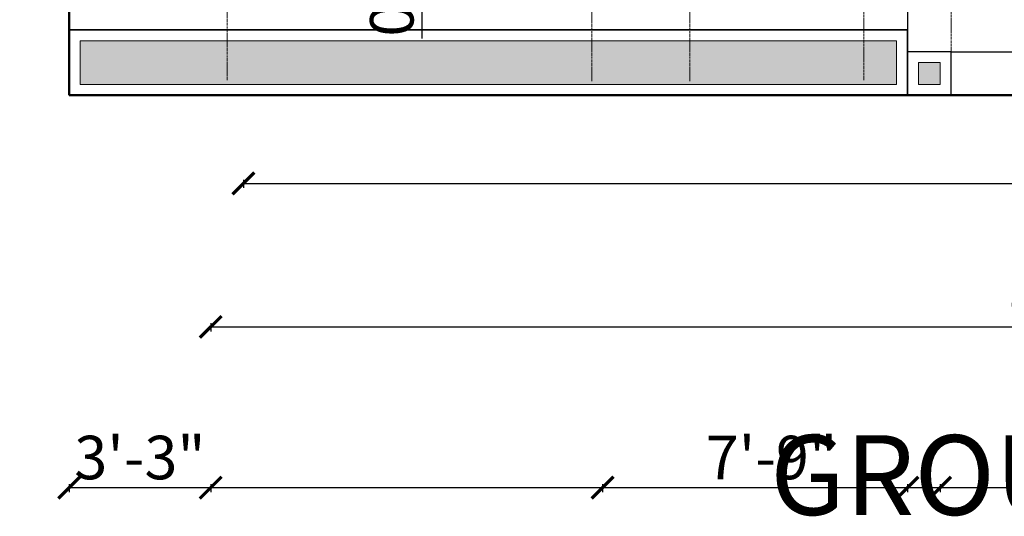
# Model space of a CAD drawing. Units: inches. Extents: x 261 to 2725, y 291 to 1454.
# Tile 2 of 35: x 417 to 688, y 296 to 433. Entities that reach past the tile are written whole.
import ezdxf

# ---------------------------------------------------------------- set-up
doc = ezdxf.new("R2010")
doc.units = ezdxf.units.IN
doc.linetypes.add('CENTER', pattern=[2, 1.25, -0.25, 0.25, -0.25])
for name, color, linetype, lineweight in [('A-ANNO-DIMS', 136, 'Continuous', 18), ('A-ANNO-TEXT', 7, 'Continuous', 25), ('A-FLOR-STRS', 42, 'Continuous', 25), ('A-GRID', 251, 'CENTER', 13), ('A-PLNT', 3, 'Continuous', 18), ('A-PLNT-PATT', 3, 'Continuous', 13), ('A-WALL', 222, 'Continuous', 50), ('C-PROP', 7, 'Continuous', 35)]:
    doc.layers.add(name, color=color, linetype=linetype, lineweight=lineweight)
doc.styles.get("Standard").update_dxf_attribs({"font": 'arial.ttf'})
doc.dimstyles.new('ISO-25', dxfattribs={"dimtxt": 12, "dimasz": 6, "dimexe": 1.25, "dimexo": 0.625, "dimtad": 1, "dimdec": 0, "dimlunit": 3, "dimtxsty": 'Standard', "dimblk": 'ARCHTICK', "dimcen": 2.5, "dimadec": 0, "dimazin": 0, "dimtfac": 1, "dimtdec": 0, "dimtmove": 0, "dimatfit": 3, "dimfxl": 1, "dimfxlon": 1, "dimarcsym": 0})

# ---------------------------------------------------------------- blocks, each defined once
blk = doc.blocks.new('_ArchTick')
at = {"color": 0, "linetype": 'ByBlock', "const_width": 0.15}
blk.add_lwpolyline([(-0.5, -0.5), (0.5, 0.5)], dxfattribs=at)
blk = doc.blocks.new('*D28')
at = {"layer": 'A-ANNO-DIMS', "color": 0, "lineweight": -2, "transparency": 16777216}
for p, q in [((469.45, 349.55), (469.45, 347.3)), ((469.45, 348.55), (955.45, 348.55)), ((955.45, 349.55), (955.45, 347.3))]:
    blk.add_line(p, q, dxfattribs=at)
at = {"layer": 'Defpoints', "color": 0, "transparency": 16777216}
for p in [(469.45, 508.47), (955.45, 508.47), (955.45, 348.55)]:
    blk.add_point(p, dxfattribs=at)
at = {"layer": 'A-ANNO-DIMS', "color": 0, "lineweight": -2, "transparency": 16777216, "xscale": 6, "yscale": 6, "zscale": 6, "rotation": 180}
blk.add_blockref('_ArchTick', (469.45, 348.55), dxfattribs=at)
at = {"layer": 'A-ANNO-DIMS', "color": 0, "lineweight": -2, "transparency": 16777216, "xscale": 6, "yscale": 6, "zscale": 6}
blk.add_blockref('_ArchTick', (955.45, 348.55), dxfattribs=at)
at = {"layer": 'A-ANNO-DIMS', "color": 0, "transparency": 16777216, "insert": (712.45, 355.3), "char_height": 12, "attachment_point": 5}
blk.add_mtext('40\'-6"', dxfattribs=at)
blk = doc.blocks.new('*D31')
at = {"layer": 'A-ANNO-DIMS', "color": 0, "lineweight": -2, "transparency": 16777216}
for p, q in [((478.45, 389.14), (478.45, 386.89)), ((478.45, 388.14), (946.45, 388.14)), ((946.45, 389.14), (946.45, 386.89))]:
    blk.add_line(p, q, dxfattribs=at)
at = {"layer": 'Defpoints', "color": 0, "transparency": 16777216}
for p in [(478.45, 517.47), (946.45, 517.47), (946.45, 388.14)]:
    blk.add_point(p, dxfattribs=at)
at = {"layer": 'A-ANNO-DIMS', "color": 0, "lineweight": -2, "transparency": 16777216, "xscale": 6, "yscale": 6, "zscale": 6, "rotation": 180}
blk.add_blockref('_ArchTick', (478.45, 388.14), dxfattribs=at)
at = {"layer": 'A-ANNO-DIMS', "color": 0, "lineweight": -2, "transparency": 16777216, "xscale": 6, "yscale": 6, "zscale": 6}
blk.add_blockref('_ArchTick', (946.45, 388.14), dxfattribs=at)
at = {"layer": 'A-ANNO-DIMS', "color": 0, "transparency": 16777216, "insert": (712.45, 394.89), "char_height": 12, "attachment_point": 5}
blk.add_mtext("39'", dxfattribs=at)
blk = doc.blocks.new('*D40')
at = {"layer": 'A-ANNO-DIMS', "color": 0, "lineweight": -2, "ltscale": 0.07, "transparency": 16777216}
for p, q in [((528.65, 517.47), (526.4, 517.47)), ((527.65, 517.47), (527.65, 508.47)), ((528.65, 508.47), (526.4, 508.47)), ((527.65, 508.47), (527.65, 428.07))]:
    blk.add_line(p, q, dxfattribs=at)
at = {"layer": 'Defpoints', "color": 0, "ltscale": 0.07, "transparency": 16777216}
for p in [(538.45, 517.47), (527.65, 508.47), (538.45, 508.47)]:
    blk.add_point(p, dxfattribs=at)
at = {"layer": 'A-ANNO-DIMS', "color": 0, "lineweight": -2, "ltscale": 0.07, "transparency": 16777216, "xscale": 6, "yscale": 6, "zscale": 6}
for p, rotation in [((527.65, 517.47), 90), ((527.65, 508.47), 270)]:
    blk.add_blockref('_ArchTick', p, dxfattribs=dict(at, rotation=rotation))
at = {"layer": 'A-ANNO-DIMS', "color": 0, "ltscale": 0.07, "transparency": 16777216, "insert": (520.9, 465.27), "char_height": 12, "attachment_point": 5, "rotation": 90}
blk.add_mtext('0\'-9" TYP.', dxfattribs=at)
blk = doc.blocks.new('*D88')
at = {"layer": 'A-ANNO-DIMS', "color": 0, "lineweight": -2, "ltscale": 0.07, "transparency": 16777216}
for p, q in [((430.45, 305.22), (430.45, 302.97)), ((430.45, 304.22), (994.45, 304.22)), ((994.45, 305.22), (994.45, 302.97))]:
    blk.add_line(p, q, dxfattribs=at)
at = {"layer": 'Defpoints', "color": 0, "ltscale": 0.07, "transparency": 16777216}
for p in [(430.45, 412.47), (994.45, 412.47), (994.45, 304.22)]:
    blk.add_point(p, dxfattribs=at)
at = {"layer": 'A-ANNO-DIMS', "color": 0, "lineweight": -2, "ltscale": 0.07, "transparency": 16777216, "xscale": 6, "yscale": 6, "zscale": 6, "rotation": 180}
blk.add_blockref('_ArchTick', (430.45, 304.22), dxfattribs=at)
at = {"layer": 'A-ANNO-DIMS', "color": 0, "lineweight": -2, "ltscale": 0.07, "transparency": 16777216, "xscale": 6, "yscale": 6, "zscale": 6}
blk.add_blockref('_ArchTick', (994.45, 304.22), dxfattribs=at)
at = {"layer": 'A-ANNO-DIMS', "color": 0, "ltscale": 0.07, "transparency": 16777216, "insert": (712.45, 310.97), "char_height": 12, "attachment_point": 5}
blk.add_mtext('47\'-0"', dxfattribs=at)
blk = doc.blocks.new('*D90')
at = {"layer": 'A-ANNO-DIMS', "color": 0, "lineweight": -2, "ltscale": 0.07, "transparency": 16777216}
for p, q in [((286.06, 430.47), (286.06, 468.49)), ((287.06, 430.47), (284.81, 430.47)), ((286.06, 412.47), (286.06, 430.47)), ((287.06, 412.47), (284.81, 412.47))]:
    blk.add_line(p, q, dxfattribs=at)
at = {"layer": 'Defpoints', "color": 0, "ltscale": 0.07, "transparency": 16777216}
for p in [(286.06, 430.47), (430.45, 430.47), (430.45, 412.47)]:
    blk.add_point(p, dxfattribs=at)
at = {"layer": 'A-ANNO-DIMS', "color": 0, "lineweight": -2, "ltscale": 0.07, "transparency": 16777216, "xscale": 6, "yscale": 6, "zscale": 6}
for p, rotation in [((286.06, 430.47), 90), ((286.06, 412.47), 270)]:
    blk.add_blockref('_ArchTick', p, dxfattribs=dict(at, rotation=rotation))
at = {"layer": 'A-ANNO-DIMS', "color": 0, "ltscale": 0.07, "transparency": 16777216, "insert": (279.3, 452.48), "char_height": 12, "attachment_point": 5, "rotation": 90}
blk.add_mtext('1\'-6"', dxfattribs=at)
blk = doc.blocks.new('*D91')
at = {"layer": 'A-ANNO-DIMS', "color": 0, "lineweight": -2, "ltscale": 0.07, "transparency": 16777216}
for p, q in [((430.45, 305.22), (430.45, 302.97)), ((430.45, 304.22), (469.45, 304.22)), ((469.45, 305.22), (469.45, 302.97))]:
    blk.add_line(p, q, dxfattribs=at)
at = {"layer": 'Defpoints', "color": 0, "ltscale": 0.07, "transparency": 16777216}
for p in [(469.45, 508.47), (430.45, 430.47), (469.45, 304.22)]:
    blk.add_point(p, dxfattribs=at)
at = {"layer": 'A-ANNO-DIMS', "color": 0, "lineweight": -2, "ltscale": 0.07, "transparency": 16777216, "xscale": 6, "yscale": 6, "zscale": 6, "rotation": 180}
blk.add_blockref('_ArchTick', (430.45, 304.22), dxfattribs=at)
at = {"layer": 'A-ANNO-DIMS', "color": 0, "lineweight": -2, "ltscale": 0.07, "transparency": 16777216, "xscale": 6, "yscale": 6, "zscale": 6}
blk.add_blockref('_ArchTick', (469.45, 304.22), dxfattribs=at)
at = {"layer": 'A-ANNO-DIMS', "color": 0, "ltscale": 0.07, "transparency": 16777216, "insert": (449.95, 310.97), "char_height": 12, "attachment_point": 5}
blk.add_mtext('3\'-3"', dxfattribs=at)
blk = doc.blocks.new('*D93')
at = {"layer": 'A-ANNO-DIMS', "color": 0, "lineweight": -2, "ltscale": 0.07, "transparency": 16777216}
for p, q in [((661.45, 305.22), (661.45, 302.97)), ((661.45, 304.22), (787.45, 304.22)), ((787.45, 305.22), (787.45, 302.97))]:
    blk.add_line(p, q, dxfattribs=at)
at = {"layer": 'Defpoints', "color": 0, "ltscale": 0.07, "transparency": 16777216}
for p in [(661.45, 430.47), (787.45, 430.47), (787.45, 304.22)]:
    blk.add_point(p, dxfattribs=at)
at = {"layer": 'A-ANNO-DIMS', "color": 0, "lineweight": -2, "ltscale": 0.07, "transparency": 16777216, "xscale": 6, "yscale": 6, "zscale": 6, "rotation": 180}
blk.add_blockref('_ArchTick', (661.45, 304.22), dxfattribs=at)
at = {"layer": 'A-ANNO-DIMS', "color": 0, "lineweight": -2, "ltscale": 0.07, "transparency": 16777216, "xscale": 6, "yscale": 6, "zscale": 6}
blk.add_blockref('_ArchTick', (787.45, 304.22), dxfattribs=at)
at = {"layer": 'A-ANNO-DIMS', "color": 0, "ltscale": 0.07, "transparency": 16777216, "insert": (724.45, 310.97), "char_height": 12, "attachment_point": 5}
blk.add_mtext('10\'-6"', dxfattribs=at)
blk = doc.blocks.new('*D96')
at = {"layer": 'A-ANNO-DIMS', "color": 0, "lineweight": -2, "ltscale": 0.07, "transparency": 16777216}
for p, q in [((577.45, 305.22), (577.45, 302.97)), ((577.45, 304.22), (670.45, 304.22)), ((670.45, 305.22), (670.45, 302.97))]:
    blk.add_line(p, q, dxfattribs=at)
at = {"layer": 'Defpoints', "color": 0, "ltscale": 0.07, "transparency": 16777216}
for p in [(577.45, 775.47), (670.45, 775.47), (670.45, 304.22)]:
    blk.add_point(p, dxfattribs=at)
at = {"layer": 'A-ANNO-DIMS', "color": 0, "lineweight": -2, "ltscale": 0.07, "transparency": 16777216, "xscale": 6, "yscale": 6, "zscale": 6, "rotation": 180}
blk.add_blockref('_ArchTick', (577.45, 304.22), dxfattribs=at)
at = {"layer": 'A-ANNO-DIMS', "color": 0, "lineweight": -2, "ltscale": 0.07, "transparency": 16777216, "xscale": 6, "yscale": 6, "zscale": 6}
blk.add_blockref('_ArchTick', (670.45, 304.22), dxfattribs=at)
at = {"layer": 'A-ANNO-DIMS', "color": 0, "ltscale": 0.07, "transparency": 16777216, "insert": (623.95, 310.97), "char_height": 12, "attachment_point": 5}
blk.add_mtext('7\'-9"', dxfattribs=at)

msp = doc.modelspace()

# ---------------------------------------------------------------- hatches: boundary and pattern name
at = {"layer": 'A-PLNT-PATT'}
h = msp.add_hatch(dxfattribs=at)
h.set_pattern_fill('GRASS', color=256, scale=0.7)
h.paths.add_polyline_path([(658.45, 427.47), (433.45, 427.47), (433.45, 415.47), (658.45, 415.47)])
h.paths.add_polyline_path([(670.45, 421.47), (664.45, 421.47), (664.45, 415.47), (670.45, 415.47)])
h.paths.add_polyline_path([(784.45, 421.47), (778.45, 421.47), (778.45, 415.47), (784.45, 415.47)])
h.paths.add_polyline_path([(991.45, 427.47), (790.45, 427.47), (790.45, 415.47), (991.45, 415.47)])
h.paths.add_polyline_path([(1439.08, 1220.47), (1252.08, 1220.47), (1252.08, 1198.47), (1417.08, 1198.47), (1417.08, 1117.47), (1439.08, 1117.47)])
h.paths.add_polyline_path([(2304.71, 1045.85), (2016.71, 1045.85), (2016.71, 805.87), (2304.71, 805.87)])
h.paths.add_polyline_path([(1267.21, 1201.68), (1431.59, 1201.68), (1431.59, 1218.76), (1267.21, 1218.76)], flags=24)
h.paths.add_polyline_path([(2089.2, 883.04), (2242.64, 883.04), (2242.64, 936.27), (2089.2, 936.27)], flags=24)

# ---------------------------------------------------------------- linework, layer by layer
at = {"layer": 'A-FLOR-STRS'}
for p, q in [((661.45, 508.47), (661.45, 412.47)), ((673.45, 424.47), (775.45, 424.47)), ((661.45, 412.47), (787.45, 412.47))]:
    msp.add_line(p, q, dxfattribs=at)
msp.add_lwpolyline([(661.45, 412.47), (673.45, 412.47), (673.45, 424.47), (661.45, 424.47)], close=True, dxfattribs=at)
at = {"layer": 'A-GRID', "ltscale": 0.5}
for p, q in [((473.95, 1330.47), (473.95, 416.47)), ((574.45, 1330.18), (574.45, 416.18)), ((601.45, 1330.18), (601.45, 416.18)), ((649.45, 1330.51), (649.45, 416.51)), ((673.45, 1330.51), (673.45, 416.51))]:
    msp.add_line(p, q, dxfattribs=at)
at = {"layer": 'A-PLNT'}
for points in [[(433.45, 415.47), (658.45, 415.47), (658.45, 427.47), (433.45, 427.47)], [(664.45, 415.47), (670.45, 415.47), (670.45, 421.47), (664.45, 421.47)]]:
    msp.add_lwpolyline(points, close=True, dxfattribs=at)
at = {"layer": 'A-WALL'}
for p, q in [((430.45, 1270.47), (430.45, 412.47)), ((430.45, 412.47), (994.45, 412.47))]:
    msp.add_line(p, q, dxfattribs=at)
at = {"layer": 'C-PROP'}
msp.add_lwpolyline([(430.45, 412.47), (661.45, 412.47), (661.45, 430.47), (430.45, 430.47)], close=True, dxfattribs=at)

# ---------------------------------------------------------------- texts
at = {"layer": 'A-ANNO-TEXT', "insert": (607.81, 318.69), "char_height": 22, "attachment_point": 1}
msp.add_mtext_dynamic_manual_height_columns('\\pxqc;{\\fTimes New Roman|b0|i0|c0|p18;GROUND FLOOR}', width=260.751, gutter_width=12.5, heights=[0], dxfattribs=at)

# ---------------------------------------------------------------- dimensions: what is measured, and where the dimension line sits
at = {"layer": 'A-ANNO-DIMS', "ltscale": 0.07}
for base, p1, p2, picture, middle in [((670.45, 304.22), (577.45, 775.47), (670.45, 775.47), '*D96', (623.95, 310.97)), ((469.45, 304.22), (430.45, 430.47), (469.45, 508.47), '*D91', (449.95, 310.97)), ((787.45, 304.22), (661.45, 430.47), (787.45, 430.47), '*D93', (724.45, 310.97)), ((994.45, 304.22), (430.45, 412.47), (994.45, 412.47), '*D88', (712.45, 310.97))]:
    dim = msp.add_linear_dim(base=base, p1=p1, p2=p2, dimstyle='ISO-25', override={"dimdec": 1, "dimlfac": 1, "dimrnd": 0, "dimzin": 1, "dimdsep": 46, "dimlunit": 4, "dimfrac": 2}, dxfattribs=at)
    dim.commit()
    dim.dimension.update_dxf_attribs({"geometry": picture, "text_midpoint": middle})
dim = msp.add_linear_dim(base=(527.65, 508.47), p1=(538.45, 517.47), p2=(538.45, 508.47), angle=270, text='<> TYP.', dimstyle='ISO-25', override={"dimdec": 1, "dimrnd": 0, "dimzin": 1, "dimlunit": 4, "dimfrac": 2}, dxfattribs=at)
dim.commit()
dim.dimension.update_dxf_attribs({"geometry": '*D40', "text_midpoint": (520.9, 465.27)})
at = {"layer": 'A-ANNO-DIMS'}
for base, p1, p2, picture, middle in [((946.45, 388.14), (478.45, 517.47), (946.45, 517.47), '*D31', (712.45, 388.14)), ((955.45, 348.55), (469.45, 508.47), (955.45, 508.47), '*D28', (712.45, 348.55))]:
    dim = msp.add_linear_dim(base=base, p1=p1, p2=p2, dimstyle='ISO-25', override={"dimclrd": 0, "dimclre": 0, "dimclrt": 0}, dxfattribs=at)
    dim.commit()
    dim.dimension.update_dxf_attribs({"geometry": picture, "text_midpoint": middle, "dimtype": 160})
at = {"layer": 'A-ANNO-DIMS', "ltscale": 0.07}
dim = msp.add_linear_dim(base=(286.06, 430.47), p1=(430.45, 412.47), p2=(430.45, 430.47), angle=90, dimstyle='ISO-25', override={"dimdec": 1, "dimlfac": 1, "dimrnd": 0, "dimzin": 1, "dimdsep": 46, "dimlunit": 4, "dimfrac": 2}, dxfattribs=at)
dim.commit()
dim.dimension.update_dxf_attribs({"geometry": '*D90', "text_midpoint": (279.3, 452.48)})

doc.saveas('drawing.dxf')
